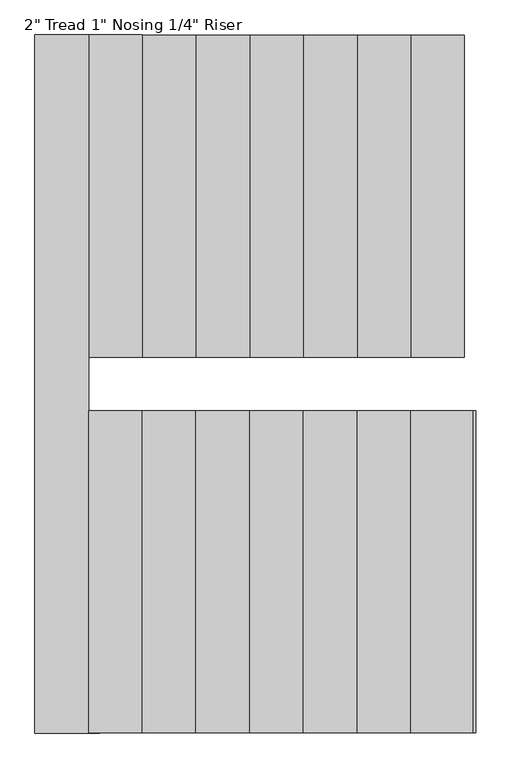
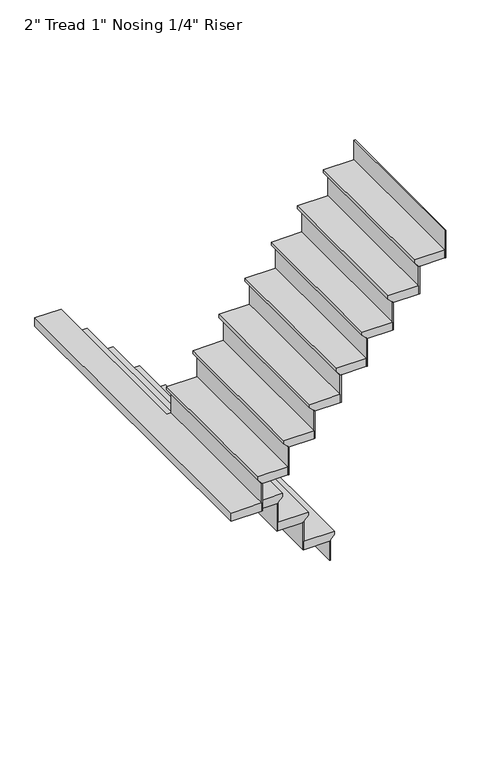
"""IFC4 building model written with IfcOpenShell, lengths in millimetres: stair flight geometry."""

from ifc_helpers import new_model, si_unit, origin, place, context, project, spatial, faceted_brep, source, transform, mapped, element, save


def stair_flight_8ca9e513(model_context):
    return source(origin(), model_context, "Body", "Brep", [
        faceted_brep([(3632.2, 10909.3, 3198.2833333), (3632.2, 10909.3, 3217.3333333), (3632.2, 9994.9, 3217.3333333), (3632.2, 9994.9, 3198.2833333), (3606.8, 10909.3, 3172.8833333), (3606.8, 9994.9, 3172.8833333), (3454.4, 10909.3, 3217.3333333), (3454.4, 9994.9, 3217.3333333), (3606.8, 9994.9, 3166.5333333), (3454.4, 9994.9, 3166.5333333), (3454.4, 10909.3, 3166.5333333), (3606.8, 10909.3, 3166.5333333)], [[[0, 1, 2, 3]], [[4, 0, 3, 5]], [[2, 1, 6, 7]], [[8, 9, 10, 11]], [[2, 7, 9, 8, 5, 3]], [[8, 11, 4, 5]], [[6, 1, 0, 4, 11, 10]], [[7, 6, 10, 9]]]),
        faceted_brep([(3606.8, 10909.3, 3166.5333333), (3606.8, 10909.3, 3048.0), (3600.45, 10909.3, 3048.0), (3600.45, 10909.3, 3166.5333333), (3606.8, 9994.9, 3166.5333333), (3600.45, 9994.9, 3166.5333333), (3600.45, 9994.9, 3048.0), (3606.8, 9994.9, 3048.0)], [[[0, 1, 2, 3]], [[4, 5, 6, 7]], [[1, 0, 4, 7]], [[2, 1, 7, 6]], [[3, 2, 6, 5]], [[0, 3, 5, 4]]]),
        faceted_brep([(3454.4, 10909.3, 3335.8666667), (3454.4, 10909.3, 3166.5333333), (3448.05, 10909.3, 3166.5333333), (3448.05, 10909.3, 3335.8666667), (3454.4, 9994.9, 3335.8666667), (3448.05, 9994.9, 3335.8666667), (3448.05, 9994.9, 3166.5333333), (3454.4, 9994.9, 3166.5333333)], [[[0, 1, 2, 3]], [[4, 5, 6, 7]], [[1, 0, 4, 7]], [[2, 1, 7, 6]], [[3, 2, 6, 5]], [[0, 3, 5, 4]]]),
        faceted_brep([(3479.8, 9994.9, 3386.6666667), (3479.8, 10909.3, 3386.6666667), (3302.0, 10909.3, 3386.6666667), (3302.0, 9994.9, 3386.6666667), (3454.4, 9994.9, 3335.8666667), (3302.0, 9994.9, 3335.8666667), (3302.0, 10909.3, 3335.8666667), (3454.4, 10909.3, 3335.8666667), (3454.4, 9994.9, 3342.2166667), (3479.8, 9994.9, 3367.6166667), (3454.4, 10909.3, 3342.2166667), (3479.8, 10909.3, 3367.6166667)], [[[0, 1, 2, 3]], [[4, 5, 6, 7]], [[0, 3, 5, 4, 8, 9]], [[4, 7, 10, 8]], [[2, 1, 11, 10, 7, 6]], [[3, 2, 6, 5]], [[11, 1, 0, 9]], [[10, 11, 9, 8]]]),
        faceted_brep([(3302.0, 10909.3, 3505.2), (3302.0, 10909.3, 3335.8666667), (3295.65, 10909.3, 3335.8666667), (3295.65, 10909.3, 3505.2), (3302.0, 9994.9, 3505.2), (3295.65, 9994.9, 3505.2), (3295.65, 9994.9, 3335.8666667), (3302.0, 9994.9, 3335.8666667)], [[[0, 1, 2, 3]], [[4, 5, 6, 7]], [[1, 0, 4, 7]], [[2, 1, 7, 6]], [[3, 2, 6, 5]], [[0, 3, 5, 4]]]),
        faceted_brep([(3327.4, 9994.9, 3556.0), (3327.4, 10909.3, 3556.0), (3149.6, 10909.3, 3556.0), (3149.6, 9994.9, 3556.0), (3302.0, 9994.9, 3505.2), (3149.6, 9994.9, 3505.2), (3149.6, 10909.3, 3505.2), (3302.0, 10909.3, 3505.2), (3302.0, 9994.9, 3511.55), (3327.4, 9994.9, 3536.95), (3302.0, 10909.3, 3511.55), (3327.4, 10909.3, 3536.95)], [[[0, 1, 2, 3]], [[4, 5, 6, 7]], [[0, 3, 5, 4, 8, 9]], [[4, 7, 10, 8]], [[2, 1, 11, 10, 7, 6]], [[3, 2, 6, 5]], [[11, 1, 0, 9]], [[10, 11, 9, 8]]]),
        faceted_brep([(3149.6, 10909.3, 3674.5333333), (3149.6, 10909.3, 3505.2), (3143.25, 10909.3, 3505.2), (3143.25, 10909.3, 3674.5333333), (3149.6, 9994.9, 3674.5333333), (3143.25, 9994.9, 3674.5333333), (3143.25, 9994.9, 3505.2), (3149.6, 9994.9, 3505.2)], [[[0, 1, 2, 3]], [[4, 5, 6, 7]], [[1, 0, 4, 7]], [[2, 1, 7, 6]], [[3, 2, 6, 5]], [[0, 3, 5, 4]]]),
        faceted_brep([(3175.0, 9994.9, 3725.3333333), (3175.0, 10909.3, 3725.3333333), (2997.2, 10909.3, 3725.3333333), (2997.2, 9994.9, 3725.3333333), (3149.6, 9994.9, 3674.5333333), (2997.2, 9994.9, 3674.5333333), (2997.2, 10909.3, 3674.5333333), (3149.6, 10909.3, 3674.5333333), (3149.6, 9994.9, 3680.8833333), (3175.0, 9994.9, 3706.2833333), (3149.6, 10909.3, 3680.8833333), (3175.0, 10909.3, 3706.2833333)], [[[0, 1, 2, 3]], [[4, 5, 6, 7]], [[0, 3, 5, 4, 8, 9]], [[4, 7, 10, 8]], [[2, 1, 11, 10, 7, 6]], [[3, 2, 6, 5]], [[11, 1, 0, 9]], [[10, 11, 9, 8]]]),
        faceted_brep([(2997.2, 10909.3, 3843.8666667), (2997.2, 10909.3, 3674.5333333), (2990.85, 10909.3, 3674.5333333), (2990.85, 10909.3, 3843.8666667), (2997.2, 9994.9, 3843.8666667), (2990.85, 9994.9, 3843.8666667), (2990.85, 9994.9, 3674.5333333), (2997.2, 9994.9, 3674.5333333)], [[[0, 1, 2, 3]], [[4, 5, 6, 7]], [[1, 0, 4, 7]], [[2, 1, 7, 6]], [[3, 2, 6, 5]], [[0, 3, 5, 4]]]),
        faceted_brep([(3022.6, 9994.9, 3894.6666667), (3022.6, 10909.3, 3894.6666667), (2844.8, 10909.3, 3894.6666667), (2844.8, 9994.9, 3894.6666667), (2997.2, 9994.9, 3843.8666667), (2844.8, 9994.9, 3843.8666667), (2844.8, 10909.3, 3843.8666667), (2997.2, 10909.3, 3843.8666667), (2997.2, 9994.9, 3850.2166667), (3022.6, 9994.9, 3875.6166667), (2997.2, 10909.3, 3850.2166667), (3022.6, 10909.3, 3875.6166667)], [[[0, 1, 2, 3]], [[4, 5, 6, 7]], [[0, 3, 5, 4, 8, 9]], [[4, 7, 10, 8]], [[2, 1, 11, 10, 7, 6]], [[3, 2, 6, 5]], [[11, 1, 0, 9]], [[10, 11, 9, 8]]]),
        faceted_brep([(2844.8, 10909.3, 4013.2), (2844.8, 10909.3, 3843.8666667), (2838.45, 10909.3, 3843.8666667), (2838.45, 10909.3, 4013.2), (2844.8, 9994.9, 4013.2), (2838.45, 9994.9, 4013.2), (2838.45, 9994.9, 3843.8666667), (2844.8, 9994.9, 3843.8666667)], [[[0, 1, 2, 3]], [[4, 5, 6, 7]], [[1, 0, 4, 7]], [[2, 1, 7, 6]], [[3, 2, 6, 5]], [[0, 3, 5, 4]]]),
        faceted_brep([(2870.2, 9994.9, 4064.0), (2870.2, 10909.3, 4064.0), (2692.4, 10909.3, 4064.0), (2692.4, 9994.9, 4064.0), (2844.8, 9994.9, 4013.2), (2692.4, 9994.9, 4013.2), (2692.4, 10909.3, 4013.2), (2844.8, 10909.3, 4013.2), (2844.8, 9994.9, 4019.55), (2870.2, 9994.9, 4044.95), (2844.8, 10909.3, 4019.55), (2870.2, 10909.3, 4044.95)], [[[0, 1, 2, 3]], [[4, 5, 6, 7]], [[0, 3, 5, 4, 8, 9]], [[4, 7, 10, 8]], [[2, 1, 11, 10, 7, 6]], [[3, 2, 6, 5]], [[11, 1, 0, 9]], [[10, 11, 9, 8]]]),
        faceted_brep([(2692.4, 10909.3, 4182.5333333), (2692.4, 10909.3, 4013.2), (2686.05, 10909.3, 4013.2), (2686.05, 10909.3, 4182.5333333), (2692.4, 9994.9, 4182.5333333), (2686.05, 9994.9, 4182.5333333), (2686.05, 9994.9, 4013.2), (2692.4, 9994.9, 4013.2)], [[[0, 1, 2, 3]], [[4, 5, 6, 7]], [[1, 0, 4, 7]], [[2, 1, 7, 6]], [[3, 2, 6, 5]], [[0, 3, 5, 4]]]),
        faceted_brep([(2717.8, 9994.9, 4233.3333333), (2717.8, 10909.3, 4233.3333333), (2540.0, 10909.3, 4233.3333333), (2540.0, 9994.9, 4233.3333333), (2692.4, 9994.9, 4182.5333333), (2540.0, 9994.9, 4182.5333333), (2540.0, 10909.3, 4182.5333333), (2692.4, 10909.3, 4182.5333333), (2692.4, 9994.9, 4188.8833333), (2717.8, 9994.9, 4214.2833333), (2692.4, 10909.3, 4188.8833333), (2717.8, 10909.3, 4214.2833333)], [[[0, 1, 2, 3]], [[4, 5, 6, 7]], [[0, 3, 5, 4, 8, 9]], [[4, 7, 10, 8]], [[2, 1, 11, 10, 7, 6]], [[3, 2, 6, 5]], [[11, 1, 0, 9]], [[10, 11, 9, 8]]]),
        faceted_brep([(2540.0, 10909.3, 4351.8666667), (2540.0, 10909.3, 4182.5333333), (2533.65, 10909.3, 4182.5333333), (2533.65, 10909.3, 4351.8666667), (2540.0, 9994.9, 4351.8666667), (2533.65, 9994.9, 4351.8666667), (2533.65, 9994.9, 4182.5333333), (2540.0, 9994.9, 4182.5333333)], [[[0, 1, 2, 3]], [[4, 5, 6, 7]], [[1, 0, 4, 7]], [[2, 1, 7, 6]], [[3, 2, 6, 5]], [[0, 3, 5, 4]]]),
        faceted_brep([(2590.8, 9842.5, 4402.6666667), (2565.4, 9842.5, 4402.6666667), (2565.4, 10909.3, 4402.6666667), (2413.0, 10909.3, 4402.6666667), (2413.0, 8928.1, 4402.6666667), (2590.8, 8928.1, 4402.6666667), (2565.4, 9842.5, 4351.8666667), (2590.8, 9842.5, 4351.8666667), (2590.8, 8928.1, 4351.8666667), (2413.0, 8928.1, 4351.8666667), (2413.0, 10909.3, 4351.8666667), (2540.0, 10909.3, 4351.8666667), (2540.0, 9994.9, 4351.8666667), (2565.4, 9994.9, 4351.8666667), (2565.4, 9994.9, 4383.6166667), (2565.4, 10909.3, 4383.6166667), (2540.0, 9994.9, 4358.2166667), (2540.0, 10909.3, 4358.2166667)], [[[0, 1, 2, 3, 4, 5]], [[6, 7, 8, 9, 10, 11, 12, 13]], [[1, 0, 7, 6]], [[2, 1, 6, 13, 14, 15]], [[13, 12, 16, 14]], [[12, 11, 17, 16]], [[3, 2, 15, 17, 11, 10]], [[4, 3, 10, 9]], [[5, 4, 9, 8]], [[0, 5, 8, 7]], [[17, 15, 14, 16]]]),
        faceted_brep([(2590.8, 8928.1, 4521.2), (2590.8, 8928.1, 4351.8666667), (2597.15, 8928.1, 4351.8666667), (2597.15, 8928.1, 4521.2), (2590.8, 9842.5, 4521.2), (2597.15, 9842.5, 4521.2), (2597.15, 9842.5, 4351.8666667), (2590.8, 9842.5, 4351.8666667)], [[[0, 1, 2, 3]], [[4, 5, 6, 7]], [[1, 0, 4, 7]], [[2, 1, 7, 6]], [[3, 2, 6, 5]], [[0, 3, 5, 4]]]),
        faceted_brep([(2565.4, 9842.5, 4572.0), (2565.4, 8928.1, 4572.0), (2743.2, 8928.1, 4572.0), (2743.2, 9842.5, 4572.0), (2590.8, 9842.5, 4521.2), (2743.2, 9842.5, 4521.2), (2743.2, 8928.1, 4521.2), (2590.8, 8928.1, 4521.2), (2590.8, 9842.5, 4527.55), (2565.4, 9842.5, 4552.95), (2590.8, 8928.1, 4527.55), (2565.4, 8928.1, 4552.95)], [[[0, 1, 2, 3]], [[4, 5, 6, 7]], [[0, 3, 5, 4, 8, 9]], [[4, 7, 10, 8]], [[2, 1, 11, 10, 7, 6]], [[3, 2, 6, 5]], [[11, 1, 0, 9]], [[10, 11, 9, 8]]]),
        faceted_brep([(2743.2, 8928.1, 4690.5333333), (2743.2, 8928.1, 4521.2), (2749.55, 8928.1, 4521.2), (2749.55, 8928.1, 4690.5333333), (2743.2, 9842.5, 4690.5333333), (2749.55, 9842.5, 4690.5333333), (2749.55, 9842.5, 4521.2), (2743.2, 9842.5, 4521.2)], [[[0, 1, 2, 3]], [[4, 5, 6, 7]], [[1, 0, 4, 7]], [[2, 1, 7, 6]], [[3, 2, 6, 5]], [[0, 3, 5, 4]]]),
        faceted_brep([(2717.8, 9842.5, 4741.3333333), (2717.8, 8928.1, 4741.3333333), (2895.6, 8928.1, 4741.3333333), (2895.6, 9842.5, 4741.3333333), (2743.2, 9842.5, 4690.5333333), (2895.6, 9842.5, 4690.5333333), (2895.6, 8928.1, 4690.5333333), (2743.2, 8928.1, 4690.5333333), (2743.2, 9842.5, 4696.8833333), (2717.8, 9842.5, 4722.2833333), (2743.2, 8928.1, 4696.8833333), (2717.8, 8928.1, 4722.2833333)], [[[0, 1, 2, 3]], [[4, 5, 6, 7]], [[0, 3, 5, 4, 8, 9]], [[4, 7, 10, 8]], [[2, 1, 11, 10, 7, 6]], [[3, 2, 6, 5]], [[11, 1, 0, 9]], [[10, 11, 9, 8]]]),
        faceted_brep([(2895.6, 8928.1, 4859.8666667), (2895.6, 8928.1, 4690.5333333), (2901.95, 8928.1, 4690.5333333), (2901.95, 8928.1, 4859.8666667), (2895.6, 9842.5, 4859.8666667), (2901.95, 9842.5, 4859.8666667), (2901.95, 9842.5, 4690.5333333), (2895.6, 9842.5, 4690.5333333)], [[[0, 1, 2, 3]], [[4, 5, 6, 7]], [[1, 0, 4, 7]], [[2, 1, 7, 6]], [[3, 2, 6, 5]], [[0, 3, 5, 4]]]),
        faceted_brep([(2870.2, 9842.5, 4910.6666667), (2870.2, 8928.1, 4910.6666667), (3048.0, 8928.1, 4910.6666667), (3048.0, 9842.5, 4910.6666667), (2895.6, 9842.5, 4859.8666667), (3048.0, 9842.5, 4859.8666667), (3048.0, 8928.1, 4859.8666667), (2895.6, 8928.1, 4859.8666667), (2895.6, 9842.5, 4866.2166667), (2870.2, 9842.5, 4891.6166667), (2895.6, 8928.1, 4866.2166667), (2870.2, 8928.1, 4891.6166667)], [[[0, 1, 2, 3]], [[4, 5, 6, 7]], [[0, 3, 5, 4, 8, 9]], [[4, 7, 10, 8]], [[2, 1, 11, 10, 7, 6]], [[3, 2, 6, 5]], [[11, 1, 0, 9]], [[10, 11, 9, 8]]]),
        faceted_brep([(3048.0, 8928.1, 5029.2), (3048.0, 8928.1, 4859.8666667), (3054.35, 8928.1, 4859.8666667), (3054.35, 8928.1, 5029.2), (3048.0, 9842.5, 5029.2), (3054.35, 9842.5, 5029.2), (3054.35, 9842.5, 4859.8666667), (3048.0, 9842.5, 4859.8666667)], [[[0, 1, 2, 3]], [[4, 5, 6, 7]], [[1, 0, 4, 7]], [[2, 1, 7, 6]], [[3, 2, 6, 5]], [[0, 3, 5, 4]]]),
        faceted_brep([(3022.6, 9842.5, 5080.0), (3022.6, 8928.1, 5080.0), (3200.4, 8928.1, 5080.0), (3200.4, 9842.5, 5080.0), (3048.0, 9842.5, 5029.2), (3200.4, 9842.5, 5029.2), (3200.4, 8928.1, 5029.2), (3048.0, 8928.1, 5029.2), (3048.0, 9842.5, 5035.55), (3022.6, 9842.5, 5060.95), (3048.0, 8928.1, 5035.55), (3022.6, 8928.1, 5060.95)], [[[0, 1, 2, 3]], [[4, 5, 6, 7]], [[0, 3, 5, 4, 8, 9]], [[4, 7, 10, 8]], [[2, 1, 11, 10, 7, 6]], [[3, 2, 6, 5]], [[11, 1, 0, 9]], [[10, 11, 9, 8]]]),
        faceted_brep([(3200.4, 8928.1, 5198.5333333), (3200.4, 8928.1, 5029.2), (3206.75, 8928.1, 5029.2), (3206.75, 8928.1, 5198.5333333), (3200.4, 9842.5, 5198.5333333), (3206.75, 9842.5, 5198.5333333), (3206.75, 9842.5, 5029.2), (3200.4, 9842.5, 5029.2)], [[[0, 1, 2, 3]], [[4, 5, 6, 7]], [[1, 0, 4, 7]], [[2, 1, 7, 6]], [[3, 2, 6, 5]], [[0, 3, 5, 4]]]),
        faceted_brep([(3175.0, 9842.5, 5249.3333333), (3175.0, 8928.1, 5249.3333333), (3352.8, 8928.1, 5249.3333333), (3352.8, 9842.5, 5249.3333333), (3200.4, 9842.5, 5198.5333333), (3352.8, 9842.5, 5198.5333333), (3352.8, 8928.1, 5198.5333333), (3200.4, 8928.1, 5198.5333333), (3200.4, 9842.5, 5204.8833333), (3175.0, 9842.5, 5230.2833333), (3200.4, 8928.1, 5204.8833333), (3175.0, 8928.1, 5230.2833333)], [[[0, 1, 2, 3]], [[4, 5, 6, 7]], [[0, 3, 5, 4, 8, 9]], [[4, 7, 10, 8]], [[2, 1, 11, 10, 7, 6]], [[3, 2, 6, 5]], [[11, 1, 0, 9]], [[10, 11, 9, 8]]]),
        faceted_brep([(3352.8, 8928.1, 5367.8666667), (3352.8, 8928.1, 5198.5333333), (3359.15, 8928.1, 5198.5333333), (3359.15, 8928.1, 5367.8666667), (3352.8, 9842.5, 5367.8666667), (3359.15, 9842.5, 5367.8666667), (3359.15, 9842.5, 5198.5333333), (3352.8, 9842.5, 5198.5333333)], [[[0, 1, 2, 3]], [[4, 5, 6, 7]], [[1, 0, 4, 7]], [[2, 1, 7, 6]], [[3, 2, 6, 5]], [[0, 3, 5, 4]]]),
        faceted_brep([(3327.4, 9842.5, 5418.6666667), (3327.4, 8928.1, 5418.6666667), (3505.2, 8928.1, 5418.6666667), (3505.2, 9842.5, 5418.6666667), (3352.8, 9842.5, 5367.8666667), (3505.2, 9842.5, 5367.8666667), (3505.2, 8928.1, 5367.8666667), (3352.8, 8928.1, 5367.8666667), (3352.8, 9842.5, 5374.2166667), (3327.4, 9842.5, 5399.6166667), (3352.8, 8928.1, 5374.2166667), (3327.4, 8928.1, 5399.6166667)], [[[0, 1, 2, 3]], [[4, 5, 6, 7]], [[0, 3, 5, 4, 8, 9]], [[4, 7, 10, 8]], [[2, 1, 11, 10, 7, 6]], [[3, 2, 6, 5]], [[11, 1, 0, 9]], [[10, 11, 9, 8]]]),
        faceted_brep([(3505.2, 8928.1, 5537.2), (3505.2, 8928.1, 5367.8666667), (3511.55, 8928.1, 5367.8666667), (3511.55, 8928.1, 5537.2), (3505.2, 9842.5, 5537.2), (3511.55, 9842.5, 5537.2), (3511.55, 9842.5, 5367.8666667), (3505.2, 9842.5, 5367.8666667)], [[[0, 1, 2, 3]], [[4, 5, 6, 7]], [[1, 0, 4, 7]], [[2, 1, 7, 6]], [[3, 2, 6, 5]], [[0, 3, 5, 4]]]),
        faceted_brep([(3657.6, 8928.1, 5706.5333333), (3657.6, 8928.1, 5537.2), (3663.95, 8928.1, 5537.2), (3663.95, 8928.1, 5706.5333333), (3657.6, 9842.5, 5706.5333333), (3663.95, 9842.5, 5706.5333333), (3663.95, 9842.5, 5537.2), (3657.6, 9842.5, 5537.2)], [[[0, 1, 2, 3]], [[4, 5, 6, 7]], [[1, 0, 4, 7]], [[2, 1, 7, 6]], [[3, 2, 6, 5]], [[0, 3, 5, 4]]]),
        faceted_brep([(3479.8, 9842.5, 5588.0), (3479.8, 8928.1, 5588.0), (3657.6, 8928.1, 5588.0), (3657.6, 9842.5, 5588.0), (3505.2, 9842.5, 5537.2), (3657.6, 9842.5, 5537.2), (3657.6, 8928.1, 5537.2), (3505.2, 8928.1, 5537.2), (3505.2, 9842.5, 5543.55), (3479.8, 9842.5, 5568.95), (3505.2, 8928.1, 5543.55), (3479.8, 8928.1, 5568.95)], [[[0, 1, 2, 3]], [[4, 5, 6, 7]], [[0, 3, 5, 4, 8, 9]], [[4, 7, 10, 8]], [[2, 1, 11, 10, 7, 6]], [[3, 2, 6, 5]], [[11, 1, 0, 9]], [[10, 11, 9, 8]]]),
    ])


if __name__ == "__main__":
    model = new_model("IFC4")
    model_context = context("Model", 3, world=origin())
    ifc_project = project(units=[si_unit("LENGTHUNIT", "METRE", prefix="MILLI")], contexts=[model_context])
    site = spatial("IfcSite", under=ifc_project)
    building = spatial("IfcBuilding", under=site)
    placement = place(None, origin())
    stair_flight_shape = stair_flight_8ca9e513(model_context)
    element("IfcStairFlight", 1, ObjectType="2\" Tread 1\" Nosing 1/4\" Riser", at=placement, inside=building, context=model_context, shape_type="MappedRepresentation", body=[
        mapped(stair_flight_shape, transform((0.0, 0.0, 0.0), x_axis=(1.0, 0.0, 0.0), y_axis=(0.0, 1.0, 0.0), z_axis=(0.0, 0.0, 1.0))),
    ])
    save(model, "model.ifc")
